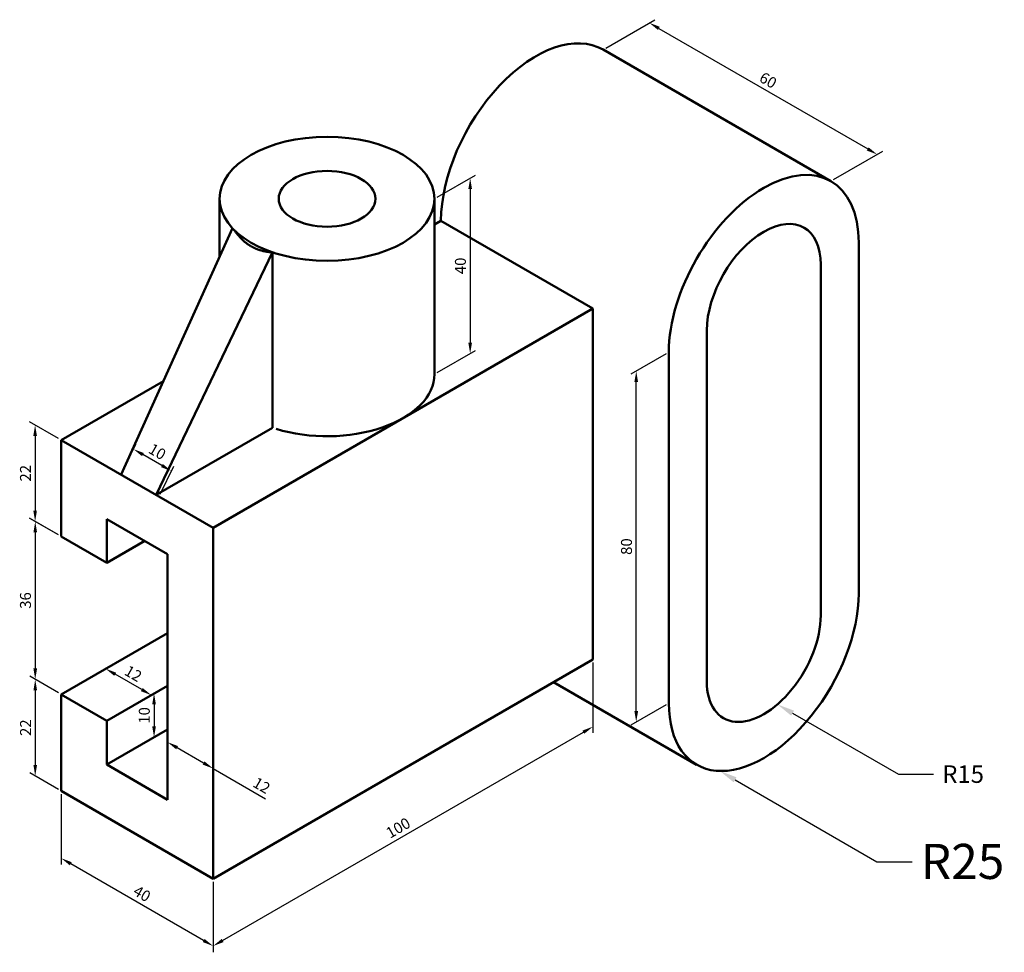
# Model space of a CAD drawing. Units: millimetres. Extents: x 1141 to 1366, y 914 to 1126.
import ezdxf
from ezdxf import colors
from ezdxf.entities.mleader import LeaderData, LeaderLine
from ezdxf.math import Vec2, Vec3

# ---------------------------------------------------------------- set-up
doc = ezdxf.new("R2010")
doc.units = ezdxf.units.MM
doc.layers.add('M-DIMS', color=2, linetype='Continuous', lineweight=25)
doc.layers.add('M-OUTL', color=7, linetype='Continuous', lineweight=50)
doc.styles.get("Standard").update_dxf_attribs({"font": 'arial.ttf'})
doc.dimstyles.new('ISO-25', dxfattribs={"dimtxt": 2.5, "dimasz": 2.5, "dimexe": 1.25, "dimexo": 0.625, "dimtad": 1, "dimtxsty": 'Standard', "dimcen": 2.5, "dimadec": 0, "dimazin": 0, "dimtfac": 1, "dimtmove": 0, "dimatfit": 3, "dimfxl": 1, "dimarcsym": 0})

# ---------------------------------------------------------------- blocks, each defined once
blk = doc.blocks.new('*D1')
at = {"layer": 'Defpoints', "color": 0, "transparency": 16777216}
for p in [(1150.74, 1030.33), (1144.79, 1011.76), (1150.74, 1008.33)]:
    blk.add_point(p, dxfattribs=at)
at = {"layer": 'M-DIMS', "color": 0, "lineweight": -2, "transparency": 16777216}
for p, q in [((1150.11, 1030.69), (1143.54, 1034.48)), ((1144.79, 1031.26), (1144.79, 1014.26)), ((1150.11, 1008.69), (1143.54, 1012.48))]:
    blk.add_line(p, q, dxfattribs=at)
at = {"layer": 'M-DIMS', "color": 0, "transparency": 16777216}
for points in [[(1144.37, 1031.26), (1145.2, 1031.26), (1144.79, 1033.76)], [(1144.37, 1014.26), (1145.2, 1014.26), (1144.79, 1011.76)]]:
    blk.add_solid(points, dxfattribs=at)
at = {"layer": 'M-DIMS', "color": 0, "transparency": 16777216, "insert": (1142.91, 1022.76), "char_height": 2.5, "attachment_point": 5, "rotation": 90}
blk.add_mtext('22', dxfattribs=at)
blk = doc.blocks.new('*D2')
at = {"layer": 'Defpoints', "color": 0, "transparency": 16777216}
for p in [(1150.74, 972.33), (1144.81, 953.75), (1150.74, 950.33)]:
    blk.add_point(p, dxfattribs=at)
at = {"layer": 'M-DIMS', "color": 0, "lineweight": -2, "transparency": 16777216}
for p, q in [((1150.11, 972.69), (1143.56, 976.47)), ((1144.81, 973.25), (1144.81, 956.25)), ((1150.11, 950.69), (1143.56, 954.47))]:
    blk.add_line(p, q, dxfattribs=at)
at = {"layer": 'M-DIMS', "color": 0, "transparency": 16777216}
for points in [[(1144.4, 973.25), (1145.23, 973.25), (1144.81, 975.75)], [(1144.4, 956.25), (1145.23, 956.25), (1144.81, 953.75)]]:
    blk.add_solid(points, dxfattribs=at)
at = {"layer": 'M-DIMS', "color": 0, "transparency": 16777216, "insert": (1142.93, 964.75), "char_height": 2.5, "attachment_point": 5, "rotation": 90}
blk.add_mtext('22', dxfattribs=at)
blk = doc.blocks.new('*D3')
at = {"layer": 'Defpoints', "color": 0, "transparency": 16777216}
for p in [(1150.74, 1008.33), (1144.81, 975.75), (1150.74, 972.33)]:
    blk.add_point(p, dxfattribs=at)
at = {"layer": 'M-DIMS', "color": 0, "lineweight": -2, "transparency": 16777216}
for p, q in [((1150.11, 1008.69), (1143.56, 1012.47)), ((1144.81, 1009.25), (1144.81, 978.25)), ((1150.11, 972.69), (1143.56, 976.47))]:
    blk.add_line(p, q, dxfattribs=at)
at = {"layer": 'M-DIMS', "color": 0, "transparency": 16777216}
for points in [[(1144.4, 1009.25), (1145.23, 1009.25), (1144.81, 1011.75)], [(1144.4, 978.25), (1145.23, 978.25), (1144.81, 975.75)]]:
    blk.add_solid(points, dxfattribs=at)
at = {"layer": 'M-DIMS', "color": 0, "transparency": 16777216, "insert": (1142.91, 993.75), "char_height": 2.5, "attachment_point": 5, "rotation": 90}
blk.add_mtext('36', dxfattribs=at)
blk = doc.blocks.new('*D4')
at = {"layer": 'Defpoints', "color": 0, "transparency": 16777216}
for p in [(1150.74, 950.33), (1150.74, 934.98), (1185.38, 930.33)]:
    blk.add_point(p, dxfattribs=at)
at = {"layer": 'M-DIMS', "color": 0, "lineweight": -2, "transparency": 16777216}
for p, q in [((1150.74, 949.6), (1150.74, 933.54)), ((1183.22, 916.23), (1152.9, 933.73)), ((1185.38, 929.6), (1185.38, 913.54))]:
    blk.add_line(p, q, dxfattribs=at)
at = {"layer": 'M-DIMS', "color": 0, "transparency": 16777216}
for points in [[(1153.11, 934.09), (1152.7, 933.37), (1150.74, 934.98)], [(1183.42, 916.59), (1183.01, 915.87), (1185.38, 914.98)]]:
    blk.add_solid(points, dxfattribs=at)
at = {"layer": 'M-DIMS', "color": 0, "transparency": 16777216, "insert": (1169.01, 926.63), "char_height": 2.5, "attachment_point": 5, "rotation": 330}
blk.add_mtext('40', dxfattribs=at)
blk = doc.blocks.new('*D5')
at = {"layer": 'Defpoints', "color": 0, "transparency": 16777216}
for p in [(1271.98, 980.33), (1271.98, 964.98), (1185.38, 930.33)]:
    blk.add_point(p, dxfattribs=at)
at = {"layer": 'M-DIMS', "color": 0, "lineweight": -2, "transparency": 16777216}
for p, q in [((1271.98, 979.6), (1271.98, 963.54)), ((1187.55, 916.23), (1269.82, 963.73)), ((1185.38, 929.6), (1185.38, 913.54))]:
    blk.add_line(p, q, dxfattribs=at)
at = {"layer": 'M-DIMS', "color": 0, "transparency": 16777216}
for points in [[(1269.61, 964.09), (1270.03, 963.37), (1271.98, 964.98)], [(1187.34, 916.59), (1187.75, 915.87), (1185.38, 914.98)]]:
    blk.add_solid(points, dxfattribs=at)
at = {"layer": 'M-DIMS', "color": 0, "transparency": 16777216, "insert": (1227.73, 941.63), "char_height": 2.5, "attachment_point": 5, "rotation": 30}
blk.add_mtext('100', dxfattribs=at)
blk = doc.blocks.new('*D6')
at = {"layer": 'Defpoints', "color": 0, "transparency": 16777216}
for p in [(1235.86, 1085.33), (1244, 1050.03), (1235.86, 1045.33)]:
    blk.add_point(p, dxfattribs=at)
at = {"layer": 'M-DIMS', "color": 0, "lineweight": -2, "transparency": 16777216}
for p, q in [((1236.48, 1085.69), (1245.25, 1090.75)), ((1244, 1087.53), (1244, 1052.53)), ((1236.48, 1045.69), (1245.25, 1050.75))]:
    blk.add_line(p, q, dxfattribs=at)
at = {"layer": 'M-DIMS', "color": 0, "transparency": 16777216}
for points in [[(1243.58, 1087.53), (1244.42, 1087.53), (1244, 1090.03)], [(1243.58, 1052.53), (1244.42, 1052.53), (1244, 1050.03)]]:
    blk.add_solid(points, dxfattribs=at)
at = {"layer": 'M-DIMS', "color": 0, "transparency": 16777216, "insert": (1242.1, 1070.03), "char_height": 2.5, "attachment_point": 5, "rotation": 90}
blk.add_mtext('40', dxfattribs=at)
blk = doc.blocks.new('*D7')
at = {"layer": 'Defpoints', "color": 0, "transparency": 16777216}
for p in [(1289.3, 1050.33), (1281.87, 1046.04), (1289.3, 970.33)]:
    blk.add_point(p, dxfattribs=at)
at = {"layer": 'M-DIMS', "color": 0, "lineweight": -2, "transparency": 16777216}
for p, q in [((1288.68, 1049.97), (1280.62, 1045.31)), ((1281.87, 968.54), (1281.87, 1043.54)), ((1288.68, 969.97), (1280.62, 965.31))]:
    blk.add_line(p, q, dxfattribs=at)
at = {"layer": 'M-DIMS', "color": 0, "transparency": 16777216}
for points in [[(1281.45, 1043.54), (1282.29, 1043.54), (1281.87, 1046.04)], [(1281.45, 968.54), (1282.29, 968.54), (1281.87, 966.04)]]:
    blk.add_solid(points, dxfattribs=at)
at = {"layer": 'M-DIMS', "color": 0, "transparency": 16777216, "insert": (1279.97, 1006.04), "char_height": 2.5, "attachment_point": 5, "rotation": 90}
blk.add_mtext('80', dxfattribs=at)
blk = doc.blocks.new('*D8')
at = {"layer": 'Defpoints', "color": 0, "transparency": 16777216}
for p in [(1274.3, 1119.34), (1336.82, 1095.44), (1326.26, 1089.34)]:
    blk.add_point(p, dxfattribs=at)
at = {"layer": 'M-DIMS', "color": 0, "lineweight": -2, "transparency": 16777216}
for p, q in [((1274.93, 1119.7), (1286.11, 1126.16)), ((1287.02, 1124.19), (1334.66, 1096.69)), ((1326.89, 1089.7), (1338.07, 1096.16))]:
    blk.add_line(p, q, dxfattribs=at)
at = {"layer": 'M-DIMS', "color": 0, "transparency": 16777216}
for points in [[(1287.23, 1124.55), (1286.82, 1123.83), (1284.86, 1125.44)], [(1334.86, 1097.05), (1334.45, 1096.33), (1336.82, 1095.44)]]:
    blk.add_solid(points, dxfattribs=at)
at = {"layer": 'M-DIMS', "color": 0, "transparency": 16777216, "insert": (1311.79, 1112.08), "char_height": 2.5, "attachment_point": 5, "rotation": 330}
blk.add_mtext('60', dxfattribs=at)
blk = doc.blocks.new('*D9')
at = {"layer": 'Defpoints', "color": 0, "transparency": 16777216}
for p in [(1160.88, 978.18), (1150.74, 972.33), (1161.13, 966.33)]:
    blk.add_point(p, dxfattribs=at)
at = {"layer": 'M-DIMS', "color": 0, "lineweight": -2, "transparency": 16777216}
for p, q in [((1151.36, 972.69), (1162.13, 978.91)), ((1169.11, 973.43), (1163.05, 976.93)), ((1161.76, 966.69), (1172.53, 972.91))]:
    blk.add_line(p, q, dxfattribs=at)
at = {"layer": 'M-DIMS', "color": 0, "transparency": 16777216}
for points in [[(1163.26, 977.29), (1162.84, 976.57), (1160.88, 978.18)], [(1169.32, 973.79), (1168.9, 973.07), (1171.28, 972.18)]]:
    blk.add_solid(points, dxfattribs=at)
at = {"layer": 'M-DIMS', "color": 0, "transparency": 16777216, "insert": (1167.02, 976.81), "char_height": 2.5, "attachment_point": 5, "rotation": 330}
blk.add_mtext('12', dxfattribs=at)
blk = doc.blocks.new('*D10')
at = {"layer": 'Defpoints', "color": 0, "transparency": 16777216}
for p in [(1161.13, 966.33), (1171.91, 962.55), (1161.13, 956.33)]:
    blk.add_point(p, dxfattribs=at)
at = {"layer": 'M-DIMS', "color": 0, "lineweight": -2, "transparency": 16777216}
for p, q in [((1161.76, 966.69), (1173.16, 973.27)), ((1171.91, 970.05), (1171.91, 965.05)), ((1161.76, 956.69), (1173.16, 963.27))]:
    blk.add_line(p, q, dxfattribs=at)
at = {"layer": 'M-DIMS', "color": 0, "transparency": 16777216}
for points in [[(1171.49, 970.05), (1172.33, 970.05), (1171.91, 972.55)], [(1171.49, 965.05), (1172.33, 965.05), (1171.91, 962.55)]]:
    blk.add_solid(points, dxfattribs=at)
at = {"layer": 'M-DIMS', "color": 0, "transparency": 16777216, "insert": (1170.01, 967.55), "char_height": 2.5, "attachment_point": 5, "rotation": 90}
blk.add_mtext('10', dxfattribs=at)
blk = doc.blocks.new('*D11')
at = {"layer": 'Defpoints', "color": 0, "transparency": 16777216}
for p in [(1185.38, 955.45), (1174.99, 948.33), (1185.38, 942.33)]:
    blk.add_point(p, dxfattribs=at)
at = {"layer": 'M-DIMS', "color": 0, "lineweight": -2, "transparency": 16777216}
for p, q in [((1174.99, 949.05), (1174.99, 962.89)), ((1177.15, 960.2), (1183.22, 956.7)), ((1185.38, 943.05), (1185.38, 956.89)), ((1185.38, 955.45), (1197.33, 948.54))]:
    blk.add_line(p, q, dxfattribs=at)
at = {"layer": 'M-DIMS', "color": 0, "transparency": 16777216}
for points in [[(1177.36, 960.56), (1176.95, 959.83), (1174.99, 961.45)], [(1183.42, 957.06), (1183.01, 956.33), (1185.38, 955.45)]]:
    blk.add_solid(points, dxfattribs=at)
at = {"layer": 'M-DIMS', "color": 0, "transparency": 16777216, "insert": (1196.29, 951.31), "char_height": 2.5, "attachment_point": 5, "rotation": 330}
blk.add_mtext('12', dxfattribs=at)
blk = doc.blocks.new('*D12')
at = {"layer": 'Defpoints', "color": 0, "transparency": 16777216}
for p in [(1167.2, 1028.26), (1164.4, 1022.44), (1173.06, 1017.44)]:
    blk.add_point(p, dxfattribs=at)
at = {"layer": 'M-DIMS', "color": 0, "lineweight": -2, "transparency": 16777216}
for p, q in [((1164.67, 1023), (1167.75, 1029.39)), ((1173.7, 1024.51), (1169.37, 1027.01)), ((1173.33, 1018), (1176.41, 1024.39))]:
    blk.add_line(p, q, dxfattribs=at)
at = {"layer": 'M-DIMS', "color": 0, "transparency": 16777216}
for points in [[(1169.58, 1027.37), (1169.16, 1026.65), (1167.2, 1028.26)], [(1173.91, 1024.87), (1173.49, 1024.15), (1175.86, 1023.26)]]:
    blk.add_solid(points, dxfattribs=at)
at = {"layer": 'M-DIMS', "color": 0, "transparency": 16777216, "insert": (1172.49, 1027.4), "char_height": 2.5, "attachment_point": 5, "rotation": 330}
blk.add_mtext('10', dxfattribs=at)

msp = doc.modelspace()

# ---------------------------------------------------------------- linework, layer by layer
at = {"layer": 'M-OUTL'}
for p, q in [((1326.264, 1089.343), (1274.302, 1119.343)), ((1186.866, 1085.326), (1186.866, 1072.191)), ((1235.856, 1085.326), (1235.856, 1045.326)), ((1237.342, 1080.326), (1235.856, 1079.468)), ((1237.342, 1080.326), (1271.983, 1060.326)), ((1164.4, 1022.44), (1189.778, 1078.639)), ((1332.605, 1075.326), (1332.605, 995.326)), ((1172.376, 1017.826), (1198.907, 1073.144)), ((1198.907, 1033.144), (1198.907, 1073.144)), ((1323.945, 1070.326), (1323.945, 990.326)), ((1185.381, 1010.326), (1271.983, 1060.326)), ((1271.983, 1060.326), (1271.983, 980.326)), ((1297.964, 1055.326), (1297.964, 975.326)), ((1289.304, 970.326), (1289.304, 1050.326)), ((1150.74, 1030.326), (1174.035, 1043.776)), ((1198.907, 1033.144), (1172.376, 1017.826)), ((1185.381, 1010.326), (1150.74, 1030.326)), ((1150.74, 1030.326), (1150.74, 1008.326)), ((1161.132, 1002.326), (1161.132, 1012.326)), ((1161.132, 1012.326), (1174.988, 1004.326)), ((1150.74, 1008.326), (1161.132, 1002.326)), ((1185.381, 930.326), (1185.381, 1010.326)), ((1161.132, 1002.326), (1169.792, 1007.326)), ((1174.988, 948.326), (1174.988, 1004.326)), ((1150.74, 972.326), (1174.988, 986.326)), ((1271.983, 980.326), (1185.381, 930.326)), ((1295.645, 956.31), (1263.015, 975.149)), ((1150.74, 950.326), (1150.74, 972.326)), ((1150.74, 972.326), (1161.132, 966.326)), ((1161.132, 966.326), (1174.988, 974.326)), ((1161.132, 966.326), (1161.132, 956.326)), ((1161.132, 956.326), (1174.988, 964.326)), ((1161.132, 956.326), (1174.988, 948.326)), ((1150.74, 950.326), (1185.381, 930.326))]:
    msp.add_line(p, q, dxfattribs=at)
msp.add_lwpolyline([(1198.907, 1073.144), (1198.797, 1073.151), (1198.687, 1073.158), (1198.577, 1073.165), (1198.467, 1073.172), (1198.358, 1073.179), (1198.248, 1073.186), (1198.138, 1073.194), (1198.031, 1073.208), (1197.923, 1073.222), (1197.816, 1073.236), (1197.709, 1073.25), (1197.601, 1073.264), (1197.494, 1073.279), (1197.387, 1073.295), (1197.283, 1073.316), (1197.178, 1073.337), (1197.073, 1073.358), (1196.969, 1073.379), (1196.864, 1073.401), (1196.759, 1073.422), (1196.656, 1073.446), (1196.554, 1073.474), (1196.452, 1073.503), (1196.35, 1073.531), (1196.248, 1073.559), (1196.146, 1073.587), (1196.044, 1073.616), (1195.944, 1073.648), (1195.845, 1073.683), (1195.746, 1073.719), (1195.647, 1073.754), (1195.548, 1073.789), (1195.449, 1073.824), (1195.35, 1073.86), (1195.253, 1073.9), (1195.157, 1073.942), (1195.061, 1073.985), (1194.965, 1074.027), (1194.869, 1074.069), (1194.773, 1074.111), (1194.677, 1074.154), (1194.584, 1074.202), (1194.491, 1074.251), (1194.398, 1074.3), (1194.305, 1074.349), (1194.212, 1074.399), (1194.12, 1074.448), (1194.027, 1074.497), (1193.937, 1074.553), (1193.848, 1074.609), (1193.758, 1074.665), (1193.669, 1074.721), (1193.579, 1074.777), (1193.49, 1074.833), (1193.401, 1074.89), (1193.315, 1074.953), (1193.228, 1075.016), (1193.142, 1075.079), (1193.056, 1075.142), (1192.97, 1075.205), (1192.884, 1075.268), (1192.799, 1075.332), (1192.716, 1075.402), (1192.634, 1075.471), (1192.551, 1075.541), (1192.469, 1075.611), (1192.386, 1075.68), (1192.303, 1075.75), (1192.222, 1075.822), (1192.143, 1075.898), (1192.065, 1075.974), (1191.986, 1076.051), (1191.907, 1076.127), (1191.828, 1076.203), (1191.749, 1076.279), (1191.672, 1076.359), (1191.597, 1076.442), (1191.521, 1076.524), (1191.446, 1076.607), (1191.371, 1076.69), (1191.296, 1076.772), (1191.22, 1076.855), (1191.148, 1076.942), (1191.077, 1077.032), (1191.005, 1077.121), (1190.934, 1077.21), (1190.862, 1077.299), (1190.791, 1077.388), (1190.72, 1077.477), (1190.652, 1077.571), (1190.584, 1077.667), (1190.517, 1077.762), (1190.449, 1077.858), (1190.382, 1077.953), (1190.314, 1078.048), (1190.247, 1078.144)], dxfattribs=at)
for centre, major_axis, start_param, end_param in [((1258.993, 1092.826), (-15.309, -26.517), 3.1415927, 5.4977871), ((1310.954, 1062.826), (-15.309, -26.517), 2.3561945, 5.4977871), ((1310.954, 1062.826), (-9.186, -15.91), 2.3561945, 5.4977871), ((1211.361, 1045.326), (-24.495, 0), 7.3614262, 9.424778), ((1310.954, 982.826), (-15.309, -26.517), 5.4977871, 8.6393798), ((1310.954, 982.826), (-9.186, -15.91), 5.4977871, 8.6393798)]:
    msp.add_ellipse(centre, major_axis=major_axis, ratio=0.5773503, start_param=start_param, end_param=end_param, dxfattribs=at)
for major_axis in [(-24.495, 0), (-11.023, 0)]:
    msp.add_ellipse((1211.361, 1085.326), major_axis=major_axis, ratio=0.5773503, dxfattribs=at)

# ---------------------------------------------------------------- dimensions: what is measured, and where the dimension line sits
at = {"layer": 'M-DIMS'}
for p1, p2, distance, picture, middle in [((1274.302, 1119.343), (1326.264, 1089.343), 10.558, '*D8', (1311.791, 1112.085)), ((1235.856, 1085.326), (1235.856, 1045.326), 8.143, '*D6', (1242.098, 1070.028)), ((1289.304, 970.326), (1289.304, 1050.326), 7.432, '*D7', (1279.97, 1006.035)), ((1150.74, 1030.326), (1150.74, 1008.326), -5.951, '*D1', (1142.908, 1022.762)), ((1173.06, 1017.44), (1164.4, 1022.44), -6.441, '*D12', (1172.485, 1027.404)), ((1150.74, 1008.326), (1150.74, 972.326), -5.928, '*D3', (1142.91, 993.749)), ((1161.132, 966.326), (1150.74, 972.326), -10.145, '*D9', (1167.021, 976.812)), ((1185.381, 930.326), (1271.983, 980.326), -13.287, '*D5', (1227.731, 941.631)), ((1150.74, 972.326), (1150.74, 950.326), -5.928, '*D2', (1142.932, 964.749)), ((1161.132, 966.326), (1161.132, 956.326), 10.777, '*D10', (1170.007, 967.548)), ((1185.381, 930.326), (1150.74, 950.326), 13.287, '*D4', (1169.011, 926.631))]:
    dim = msp.add_aligned_dim(p1=p1, p2=p2, distance=distance, dimstyle='ISO-25', override={"dimclrd": 0, "dimclre": 0, "dimclrt": 0}, dxfattribs=at)
    dim.commit()
    dim.dimension.update_dxf_attribs({"geometry": picture, "text_midpoint": middle})
dim = msp.add_linear_dim(base=(1185.381, 955.445), p1=(1174.988, 948.326), p2=(1185.381, 942.326), angle=330, dimstyle='ISO-25', override={"dimclrd": 0, "dimclre": 0, "dimclrt": 0}, dxfattribs=at)
dim.commit()
dim.dimension.update_dxf_attribs({"geometry": '*D11', "text_midpoint": (1195.355, 949.687), "dimtype": 161})

# ---------------------------------------------------------------- leaders
ml = msp.add_multileader_mtext('Standard', dxfattribs=at)
ml.set_content('R15', color=256)
ml.set_leader_properties()
ml.build(insert=Vec2(0, 0))
ctx = ml.context
ctx.base_point, ctx.plane_origin = Vec3(1349.651, 954.133), Vec3(1314.066, 970.06)
notes = []
notes.append((ctx, [(0, (1, 1, 0), (1341.651, 954.133), (1, 0), 8, [(0, [(1314.066, 970.06)], 0, [])])]))
ctx.mtext.insert, ctx.mtext.flow_direction = Vec3(1351.651, 956.168), 5
ml = msp.add_multileader_mtext('Standard', dxfattribs=at)
ml.set_content('R25', color=256)
ml.set_leader_properties()
ml.build(insert=Vec2(0, 0))
ctx = ml.context
ctx.base_point, ctx.char_height, ctx.plane_origin = Vec3(1344.763, 934.196), 8, Vec3(1300.938, 954.88)
notes.append((ctx, [(0, (1, 1, 0), (1336.763, 934.196), (1, 0), 8, [(0, [(1300.938, 954.88)], 0, [])])]))
ctx.mtext.insert, ctx.mtext.flow_direction = Vec3(1346.763, 938.264), 5
for ctx, leaders in notes:
    for number, flags, end, landing, length, lines in leaders:
        leader = LeaderData()
        leader.index, (leader.has_last_leader_line, leader.has_dogleg_vector, leader.attachment_direction) = number, flags
        leader.last_leader_point, leader.dogleg_vector, leader.dogleg_length = Vec3(end), Vec3(landing), length
        for number, points, colour, breaks in lines:
            line = LeaderLine()
            line.index, line.vertices, line.color, line.breaks = number, Vec3.list(points), colors.encode_raw_color(colour), breaks
            leader.lines.append(line)
        ctx.leaders.append(leader)

doc.saveas('drawing.dxf')
